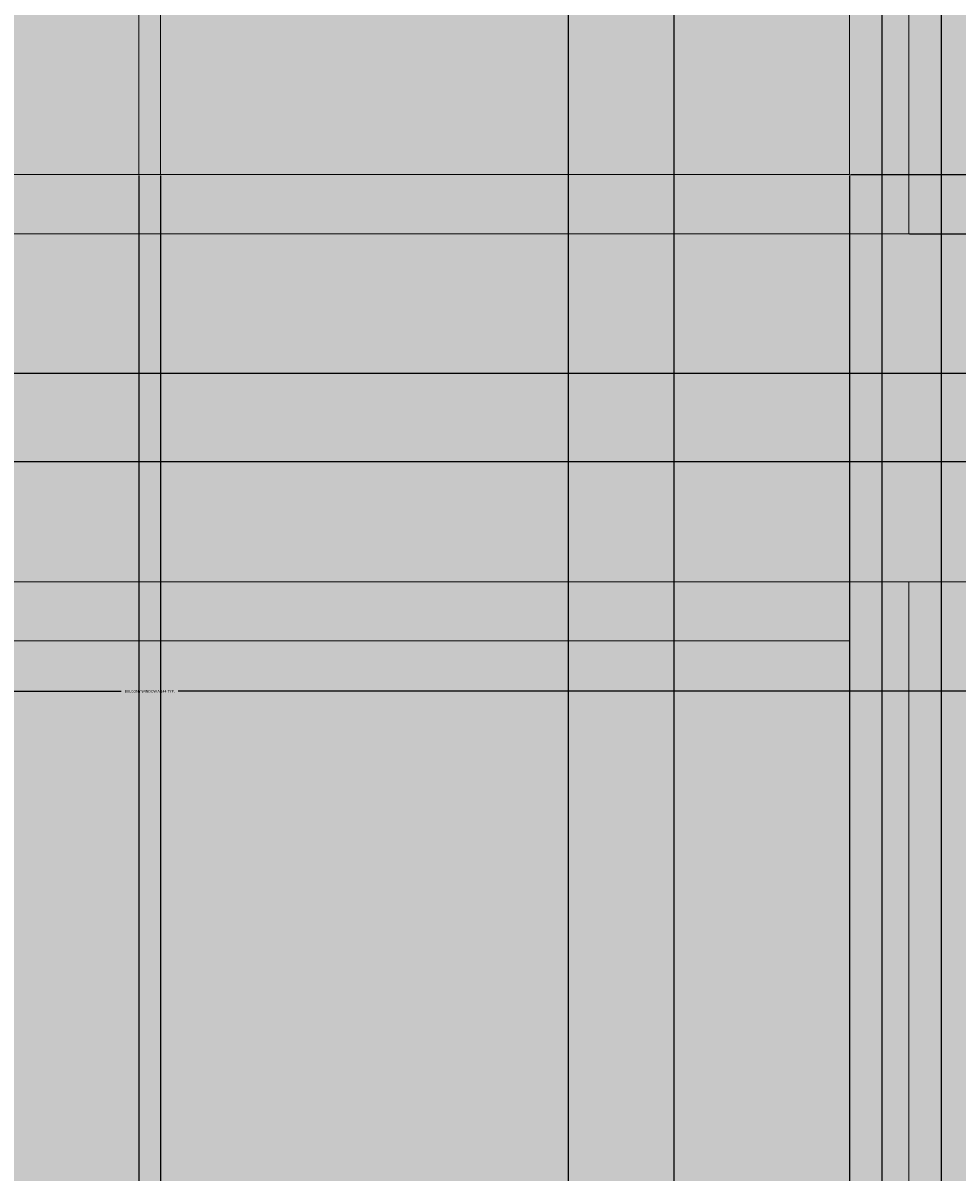
# Model space of a CAD drawing. Units: inches. Extents: x 3024 to 4744, y 1110 to 2100.
# Tile 21 of 29: x 3212 to 3275, y 1731 to 1809. Entities that reach past the tile are written whole.
import ezdxf

# ---------------------------------------------------------------- set-up
doc = ezdxf.new("R2010")
doc.units = ezdxf.units.IN
for name, color, linetype, lineweight in [('A-ANNO-DIMS', 2, 'Continuous', 18), ('A-ELEV', 7, 'Continuous', 25), ('A-ELEV-PATT', 252, 'Continuous', 13), ('A-GLAZ', 4, 'Continuous', 18)]:
    doc.layers.add(name, color=color, linetype=linetype, lineweight=lineweight)
doc.styles.get("Standard").update_dxf_attribs({"font": 'arial.ttf'})
doc.dimstyles.get("Standard").update_dxf_attribs({"dimtxt": 0.18, "dimasz": 0.18, "dimexe": 0.18, "dimexo": 0.0625, "dimgap": 0.09, "dimtad": 0, "dimtih": 1, "dimtoh": 1, "dimdec": 1, "dimzin": 0, "dimdsep": 46, "dimlunit": 3, "dimtxsty": 'Standard', "dimcen": 0.09, "dimadec": 0, "dimazin": 0, "dimtfac": 1, "dimtdec": 1, "dimtofl": 0, "dimtmove": 0, "dimatfit": 3, "dimfxl": 1, "dimtolj": 1, "dimtzin": 0, "dimarcsym": 0})

# ---------------------------------------------------------------- blocks, each defined once
blk = doc.blocks.new('WIN-BALCONY-A')
for p, q in [((3169.396, 1897.488), (3292.605, 1897.488)), ((3169.396, 1897.488), (3292.605, 1897.488)), ((3169.396, 1795.043), (3292.605, 1795.043)), ((3169.396, 1795.043), (3292.605, 1795.043))]:
    blk.add_line(p, q)
for points in [[(3148.969, 1897.488), (3148.969, 1905.611), (3292.605, 1905.611), (3292.605, 1897.488)], [(3148.969, 1897.488), (3148.969, 1905.611), (3292.605, 1905.611), (3292.605, 1897.488)], [(3292.605, 1795.043), (3292.605, 1785.611), (3148.969, 1785.611), (3148.969, 1795.043)], [(3292.605, 1795.043), (3292.605, 1785.611), (3148.969, 1785.611), (3148.969, 1795.043)]]:
    blk.add_lwpolyline(points)
for points in [[(3272.178, 1795.043), (3169.396, 1795.043), (3169.396, 1897.488), (3272.178, 1897.488)], [(3272.178, 1795.043), (3169.396, 1795.043), (3169.396, 1897.488), (3272.178, 1897.488)], [(3268.178, 1799.043), (3173.396, 1799.043), (3173.396, 1893.488), (3268.178, 1893.488)], [(3268.178, 1799.043), (3173.396, 1799.043), (3173.396, 1893.488), (3268.178, 1893.488)], [(3220.05, 1893.488), (3221.524, 1893.488), (3221.524, 1799.043), (3220.05, 1799.043)], [(3220.05, 1893.488), (3221.524, 1893.488), (3221.524, 1799.043), (3220.05, 1799.043)]]:
    blk.add_lwpolyline(points, close=True)
blk = doc.blocks.new('*D6')
at = {"layer": 'A-ANNO-DIMS', "color": 0, "lineweight": -2, "transparency": 16777216}
for p, q in [((3148.969, 1785.549), (3148.969, 1763.886)), ((3292.605, 1785.549), (3292.605, 1763.886)), ((3149.149, 1764.066), (3218.852, 1764.066)), ((3292.425, 1764.066), (3222.723, 1764.066))]:
    blk.add_line(p, q, dxfattribs=at)
at = {"layer": 'A-ANNO-DIMS', "color": 0, "transparency": 16777216}
for points in [[(3149.149, 1764.096), (3149.149, 1764.036), (3148.969, 1764.066)], [(3292.425, 1764.096), (3292.425, 1764.036), (3292.605, 1764.066)]]:
    blk.add_solid(points, dxfattribs=at)
at = {"layer": 'Defpoints', "color": 0, "transparency": 16777216}
for p in [(3148.969, 1785.611), (3292.605, 1785.611), (3292.605, 1764.066)]:
    blk.add_point(p, dxfattribs=at)
at = {"layer": 'A-ANNO-DIMS', "color": 0, "transparency": 16777216, "insert": (3220.787, 1764.066), "char_height": 0.18, "attachment_point": 5}
blk.add_mtext('\\A1;BALCONY WINDOW A 144 TYP.', dxfattribs=at)
blk = doc.blocks.new('*D64')
at = {"layer": 'A-ANNO-DIMS', "color": 0, "lineweight": -2, "transparency": 16777216}
for p, q in [((3069.794, 1241.497), (3069.794, 2100.438)), ((3741.151, 1241.497), (3741.151, 2100.438)), ((3069.974, 2100.258), (3405.078, 2100.258)), ((3740.971, 2100.258), (3405.866, 2100.258))]:
    blk.add_line(p, q, dxfattribs=at)
at = {"layer": 'A-ANNO-DIMS', "color": 0, "transparency": 16777216}
for points in [[(3069.974, 2100.288), (3069.974, 2100.228), (3069.794, 2100.258)], [(3740.971, 2100.288), (3740.971, 2100.228), (3741.151, 2100.258)]]:
    blk.add_solid(points, dxfattribs=at)
at = {"layer": 'Defpoints', "color": 0, "transparency": 16777216}
for p in [(3741.151, 2100.258), (3069.794, 1241.434), (3741.151, 1241.434)]:
    blk.add_point(p, dxfattribs=at)
at = {"layer": 'A-ANNO-DIMS', "color": 0, "transparency": 16777216, "insert": (3405.472, 2100.258), "char_height": 0.18, "attachment_point": 5}
blk.add_mtext('\\A1;671.4', dxfattribs=at)
blk = doc.blocks.new('*D91')
at = {"layer": 'A-ANNO-DIMS', "color": 0, "lineweight": -2, "transparency": 16777216}
for p, q in [((3173.396, 1798.981), (3173.396, 1109.931)), ((3220.05, 1798.981), (3220.05, 1109.931)), ((3173.576, 1110.111), (3196.325, 1110.111)), ((3219.87, 1110.111), (3197.121, 1110.111))]:
    blk.add_line(p, q, dxfattribs=at)
at = {"layer": 'A-ANNO-DIMS', "color": 0, "transparency": 16777216}
for points in [[(3173.576, 1110.141), (3173.576, 1110.081), (3173.396, 1110.111)], [(3219.87, 1110.141), (3219.87, 1110.081), (3220.05, 1110.111)]]:
    blk.add_solid(points, dxfattribs=at)
at = {"layer": 'Defpoints', "color": 0, "transparency": 16777216}
for p in [(3173.396, 1799.043), (3220.05, 1799.043), (3220.05, 1110.111)]:
    blk.add_point(p, dxfattribs=at)
at = {"layer": 'A-ANNO-DIMS', "color": 0, "transparency": 16777216, "insert": (3196.723, 1110.111), "char_height": 0.18, "attachment_point": 5}
blk.add_mtext('\\A1;46.65', dxfattribs=at)
blk = doc.blocks.new('*D92')
at = {"layer": 'A-ANNO-DIMS', "color": 0, "lineweight": -2, "transparency": 16777216}
for p, q in [((3220.05, 1798.981), (3220.05, 1109.931)), ((3221.524, 1798.981), (3221.524, 1109.931)), ((3220.23, 1110.111), (3220.472, 1110.111)), ((3221.344, 1110.111), (3221.103, 1110.111))]:
    blk.add_line(p, q, dxfattribs=at)
at = {"layer": 'A-ANNO-DIMS', "color": 0, "transparency": 16777216}
for points in [[(3220.23, 1110.141), (3220.23, 1110.081), (3220.05, 1110.111)], [(3221.344, 1110.141), (3221.344, 1110.081), (3221.524, 1110.111)]]:
    blk.add_solid(points, dxfattribs=at)
at = {"layer": 'Defpoints', "color": 0, "transparency": 16777216}
for p in [(3220.05, 1799.043), (3221.524, 1799.043), (3221.524, 1110.111)]:
    blk.add_point(p, dxfattribs=at)
at = {"layer": 'A-ANNO-DIMS', "color": 0, "transparency": 16777216, "insert": (3220.787, 1110.111), "char_height": 0.18, "attachment_point": 5}
blk.add_mtext('\\A1;1.47', dxfattribs=at)
blk = doc.blocks.new('*D93')
at = {"layer": 'A-ANNO-DIMS', "color": 0, "lineweight": -2, "transparency": 16777216}
for p, q in [((3221.524, 1798.981), (3221.524, 1109.931)), ((3268.178, 1798.981), (3268.178, 1109.931)), ((3221.704, 1110.111), (3244.453, 1110.111)), ((3267.998, 1110.111), (3245.249, 1110.111))]:
    blk.add_line(p, q, dxfattribs=at)
at = {"layer": 'A-ANNO-DIMS', "color": 0, "transparency": 16777216}
for points in [[(3221.704, 1110.141), (3221.704, 1110.081), (3221.524, 1110.111)], [(3267.998, 1110.141), (3267.998, 1110.081), (3268.178, 1110.111)]]:
    blk.add_solid(points, dxfattribs=at)
at = {"layer": 'Defpoints', "color": 0, "transparency": 16777216}
for p in [(3221.524, 1799.043), (3268.178, 1799.043), (3268.178, 1110.111)]:
    blk.add_point(p, dxfattribs=at)
at = {"layer": 'A-ANNO-DIMS', "color": 0, "transparency": 16777216, "insert": (3244.851, 1110.111), "char_height": 0.18, "attachment_point": 5}
blk.add_mtext('\\A1;46.65', dxfattribs=at)
blk = doc.blocks.new('*D100')
at = {"layer": 'A-ANNO-DIMS', "color": 0, "lineweight": -2, "transparency": 16777216}
for p, q in [((3268.241, 1799.043), (3786.831, 1799.043)), ((3786.651, 1798.863), (3786.651, 1797.225)), ((3786.651, 1795.223), (3786.651, 1796.861)), ((3272.241, 1795.043), (3786.831, 1795.043))]:
    blk.add_line(p, q, dxfattribs=at)
at = {"layer": 'A-ANNO-DIMS', "color": 0, "transparency": 16777216}
for points in [[(3786.621, 1798.863), (3786.681, 1798.863), (3786.651, 1799.043)], [(3786.621, 1795.223), (3786.681, 1795.223), (3786.651, 1795.043)]]:
    blk.add_solid(points, dxfattribs=at)
at = {"layer": 'Defpoints', "color": 0, "transparency": 16777216}
for p in [(3268.178, 1799.043), (3786.651, 1799.043), (3272.178, 1795.043)]:
    blk.add_point(p, dxfattribs=at)
at = {"layer": 'A-ANNO-DIMS', "color": 0, "transparency": 16777216, "insert": (3786.651, 1797.043), "char_height": 0.18, "attachment_point": 5}
blk.add_mtext('\\A1;4.00', dxfattribs=at)
blk = doc.blocks.new('*D101')
at = {"layer": 'A-ANNO-DIMS', "color": 0, "lineweight": -2, "transparency": 16777216}
for p, q in [((3268.241, 1893.488), (3786.831, 1893.488)), ((3786.651, 1893.308), (3786.651, 1846.447)), ((3786.651, 1799.223), (3786.651, 1846.084)), ((3268.241, 1799.043), (3786.831, 1799.043))]:
    blk.add_line(p, q, dxfattribs=at)
at = {"layer": 'A-ANNO-DIMS', "color": 0, "transparency": 16777216}
for points in [[(3786.621, 1893.308), (3786.681, 1893.308), (3786.651, 1893.488)], [(3786.621, 1799.223), (3786.681, 1799.223), (3786.651, 1799.043)]]:
    blk.add_solid(points, dxfattribs=at)
at = {"layer": 'Defpoints', "color": 0, "transparency": 16777216}
for p in [(3268.178, 1893.488), (3786.651, 1893.488), (3268.178, 1799.043)]:
    blk.add_point(p, dxfattribs=at)
at = {"layer": 'A-ANNO-DIMS', "color": 0, "transparency": 16777216, "insert": (3786.651, 1846.265), "char_height": 0.18, "attachment_point": 5}
blk.add_mtext('\\A1;94.44', dxfattribs=at)
blk = doc.blocks.new('*D107')
at = {"layer": 'A-ANNO-DIMS', "color": 0, "lineweight": -2, "transparency": 16777216}
for p, q in [((3174.161, 1271.674), (3174.161, 2100.438)), ((3270.388, 1271.674), (3270.388, 2100.438)), ((3174.341, 2100.258), (3221.881, 2100.258)), ((3270.208, 2100.258), (3222.668, 2100.258))]:
    blk.add_line(p, q, dxfattribs=at)
at = {"layer": 'A-ANNO-DIMS', "color": 0, "transparency": 16777216}
for points in [[(3174.341, 2100.288), (3174.341, 2100.228), (3174.161, 2100.258)], [(3270.208, 2100.288), (3270.208, 2100.228), (3270.388, 2100.258)]]:
    blk.add_solid(points, dxfattribs=at)
at = {"layer": 'Defpoints', "color": 0, "transparency": 16777216}
for p in [(3270.388, 2100.258), (3174.161, 1271.611), (3270.388, 1271.611)]:
    blk.add_point(p, dxfattribs=at)
at = {"layer": 'A-ANNO-DIMS', "color": 0, "transparency": 16777216, "insert": (3222.274, 2100.258), "char_height": 0.18, "attachment_point": 5}
blk.add_mtext('\\A1;96.23', dxfattribs=at)
blk = doc.blocks.new('*D108')
at = {"layer": 'A-ANNO-DIMS', "color": 0, "lineweight": -2, "transparency": 16777216}
for p, q in [((3270.388, 1271.674), (3270.388, 2100.438)), ((3274.388, 1275.674), (3274.388, 2100.438)), ((3270.568, 2100.258), (3272.061, 2100.258)), ((3274.208, 2100.258), (3272.715, 2100.258))]:
    blk.add_line(p, q, dxfattribs=at)
at = {"layer": 'A-ANNO-DIMS', "color": 0, "transparency": 16777216}
for points in [[(3270.568, 2100.288), (3270.568, 2100.228), (3270.388, 2100.258)], [(3274.208, 2100.288), (3274.208, 2100.228), (3274.388, 2100.258)]]:
    blk.add_solid(points, dxfattribs=at)
at = {"layer": 'Defpoints', "color": 0, "transparency": 16777216}
for p in [(3274.388, 2100.258), (3274.388, 1275.611), (3270.388, 1271.611)]:
    blk.add_point(p, dxfattribs=at)
at = {"layer": 'A-ANNO-DIMS', "color": 0, "transparency": 16777216, "insert": (3272.388, 2100.258), "char_height": 0.18, "attachment_point": 5}
blk.add_mtext('\\A1;4.00', dxfattribs=at)
blk = doc.blocks.new('*D126')
at = {"layer": 'A-ANNO-DIMS', "color": 0, "lineweight": -2, "transparency": 16777216}
for p, q in [((3249.143, 1256.29), (3249.143, 2100.438)), ((3256.29, 1256.29), (3256.29, 2100.438)), ((3249.323, 2100.258), (3252.324, 2100.258)), ((3256.11, 2100.258), (3253.11, 2100.258))]:
    blk.add_line(p, q, dxfattribs=at)
at = {"layer": 'A-ANNO-DIMS', "color": 0, "transparency": 16777216}
for points in [[(3249.323, 2100.288), (3249.323, 2100.228), (3249.143, 2100.258)], [(3256.11, 2100.288), (3256.11, 2100.228), (3256.29, 2100.258)]]:
    blk.add_solid(points, dxfattribs=at)
at = {"layer": 'Defpoints', "color": 0, "transparency": 16777216}
for p in [(3256.29, 2100.258), (3249.143, 1256.228), (3256.29, 1256.228)]:
    blk.add_point(p, dxfattribs=at)
at = {"layer": 'A-ANNO-DIMS', "color": 0, "transparency": 16777216, "insert": (3252.717, 2100.258), "char_height": 0.18, "attachment_point": 5}
blk.add_mtext('\\A1;7.147', dxfattribs=at)

msp = doc.modelspace()

# ---------------------------------------------------------------- hatches: boundary and pattern name
at = {"layer": 'A-ELEV-PATT'}
h = msp.add_hatch(color=256, dxfattribs=at)
h.dxf.hatch_style = 1
h.paths.add_polyline_path([(3491.8271, 2054.7584), (3320.5658, 2054.7584), (3320.5658, 2043.5286), (3491.8271, 2043.5286)])
h.paths.add_polyline_path([(3292.6051, 1905.6112), (3148.9694, 1905.6112), (3148.9694, 1897.4879), (3169.3964, 1897.4879), (3292.6051, 1897.4879)])
h.paths.add_polyline_path([(3292.6051, 1795.0431), (3169.3964, 1795.0431), (3148.9694, 1795.0431), (3148.9694, 1785.6112), (3292.6051, 1785.6112)])
h.paths.add_polyline_path([(3292.6051, 1779.6112), (3148.9694, 1779.6112), (3148.9694, 1771.4879), (3169.3964, 1771.4879), (3292.6051, 1771.4879)])
h.paths.add_polyline_path([(3292.6051, 1669.0431), (3169.3964, 1669.0431), (3148.9694, 1669.0431), (3148.9694, 1659.6112), (3292.6051, 1659.6112)])
h.paths.add_polyline_path([(3292.6051, 1653.6112), (3148.9694, 1653.6112), (3148.9694, 1645.4879), (3169.3964, 1645.4879), (3292.6051, 1645.4879)])
h.paths.add_polyline_path([(3292.6051, 1543.0431), (3169.3964, 1543.0431), (3148.9694, 1543.0431), (3148.9694, 1533.6112), (3292.6051, 1533.6112)])
h.paths.add_polyline_path([(3292.6051, 1527.6112), (3148.9694, 1527.6112), (3148.9694, 1519.4879), (3169.3964, 1519.4879), (3292.6051, 1519.4879)])
h.paths.add_polyline_path([(3292.6051, 1401.6112), (3148.9694, 1401.6112), (3148.9694, 1393.4879), (3169.3964, 1393.4879), (3292.6051, 1393.4879)])
h.paths.add_polyline_path([(3292.6051, 1417.0431), (3169.3964, 1417.0431), (3148.9694, 1417.0431), (3148.9694, 1407.6112), (3292.6051, 1407.6112)])
h.paths.add_polyline_path([(3292.6051, 1291.0431), (3169.3964, 1291.0431), (3148.9694, 1291.0431), (3148.9694, 1281.6112), (3292.6051, 1281.6112)])
h.paths.add_polyline_path([(3654.037, 1165.0431), (3530.8283, 1165.0431), (3510.4013, 1165.0431), (3510.4013, 1155.6112), (3654.037, 1155.6112)])
h.paths.add_polyline_path([(3654.037, 1275.6112), (3510.4013, 1275.6112), (3510.4013, 1267.4879), (3530.8283, 1267.4879), (3654.037, 1267.4879)])
h.paths.add_polyline_path([(3654.037, 1291.0431), (3530.8283, 1291.0431), (3510.4013, 1291.0431), (3510.4013, 1281.6112), (3654.037, 1281.6112)])
h.paths.add_polyline_path([(3654.037, 1417.0431), (3530.8283, 1417.0431), (3510.4013, 1417.0431), (3510.4013, 1407.6112), (3654.037, 1407.6112)])
h.paths.add_polyline_path([(3654.037, 1401.6112), (3510.4013, 1401.6112), (3510.4013, 1393.4879), (3530.8283, 1393.4879), (3654.037, 1393.4879)])
h.paths.add_polyline_path([(3654.037, 1543.0431), (3530.8283, 1543.0431), (3510.4013, 1543.0431), (3510.4013, 1533.6112), (3654.037, 1533.6112)])
h.paths.add_polyline_path([(3654.037, 1527.6112), (3510.4013, 1527.6112), (3510.4013, 1519.4879), (3530.8283, 1519.4879), (3654.037, 1519.4879)])
h.paths.add_polyline_path([(3654.037, 1653.6112), (3510.4013, 1653.6112), (3510.4013, 1645.4879), (3530.8283, 1645.4879), (3654.037, 1645.4879)])
h.paths.add_polyline_path([(3654.037, 1669.0431), (3530.8283, 1669.0431), (3510.4013, 1669.0431), (3510.4013, 1659.6112), (3654.037, 1659.6112)])
h.paths.add_polyline_path([(3654.037, 1779.6112), (3510.4013, 1779.6112), (3510.4013, 1771.4879), (3530.8283, 1771.4879), (3654.037, 1771.4879)])
h.paths.add_polyline_path([(3654.037, 1795.0431), (3530.8283, 1795.0431), (3510.4013, 1795.0431), (3510.4013, 1785.6112), (3654.037, 1785.6112)])
h.paths.add_polyline_path([(3654.037, 1905.6112), (3510.4013, 1905.6112), (3510.4013, 1897.4879), (3530.8283, 1897.4879), (3654.037, 1897.4879)])
h = msp.add_hatch(color=256, dxfattribs=at)
h.dxf.hatch_style = 1
h.paths.add_polyline_path([(3221.5241, 2019.4879), (3220.0505, 2019.4879), (3220.0505, 1925.0431), (3221.5241, 1925.0431)], flags=0)
h.paths.add_polyline_path([(3221.5241, 2019.4879), (3221.5241, 1925.0431), (3220.0505, 1925.0431), (3220.0505, 2019.4879)], flags=0)
h.paths.add_polyline_path([(3221.5241, 1893.4879), (3220.0505, 1893.4879), (3220.0505, 1799.0431), (3221.5241, 1799.0431)])
h = msp.add_hatch(color=256, dxfattribs=at)
h.dxf.hatch_style = 1
h.paths.add_polyline_path([(3329.7033, 1407.6112), (3105.4722, 1407.6112), (3105.4722, 1401.6112), (3329.7033, 1401.6112)])
h.paths.add_polyline_path([(3329.7033, 1281.6112), (3105.4722, 1281.6112), (3105.4722, 1275.6112), (3112.3838, 1275.6112), (3329.7033, 1275.6112)])
h.paths.add_polyline_path([(3329.7033, 1533.6112), (3105.4722, 1533.6112), (3105.4722, 1527.6112), (3329.7033, 1527.6112)])
h.paths.add_polyline_path([(3329.7033, 1659.6112), (3105.4722, 1659.6112), (3105.4722, 1653.6112), (3329.7033, 1653.6112)])
h.paths.add_polyline_path([(3329.7033, 1785.6112), (3105.4722, 1785.6112), (3105.4722, 1779.6112), (3329.7033, 1779.6112)])
h.paths.add_polyline_path([(3329.7033, 1911.6112), (3105.4722, 1911.6112), (3095.7158, 1911.6112), (3095.7158, 1905.6112), (3329.7033, 1905.6112)])
h.paths.add_polyline_path([(3715.2286, 1911.6112), (3705.4722, 1911.6112), (3705.4722, 1905.6112), (3715.2286, 1905.6112)])
h.paths.add_polyline_path([(3688.5588, 1911.6112), (3481.2411, 1911.6112), (3481.2411, 1905.6112), (3688.5588, 1905.6112)])
h = msp.add_hatch(color=256, dxfattribs=at)
h.dxf.hatch_style = 1
h.paths.add_polyline_path([(3169.3964, 1897.4879), (3160.8586, 1897.4879), (3160.8586, 1806.8674), (3163.5269, 1806.8674), (3163.5269, 1795.0431), (3169.3964, 1795.0431)])
h.paths.add_polyline_path([(3280.716, 1897.4879), (3272.1781, 1897.4879), (3272.1781, 1795.0431), (3276.5094, 1795.0431), (3276.5094, 1806.8674), (3280.716, 1806.8674)])
h.paths.add_polyline_path([(3280.716, 1771.4879), (3272.1781, 1771.4879), (3272.1781, 1669.0431), (3276.5094, 1669.0431), (3276.5094, 1680.8674), (3280.716, 1680.8674)])
h.paths.add_polyline_path([(3169.3964, 1771.4879), (3160.8586, 1771.4879), (3160.8586, 1680.8674), (3163.5269, 1680.8674), (3163.5269, 1669.0431), (3169.3964, 1669.0431)])
h.paths.add_polyline_path([(3169.3964, 1645.4879), (3160.8586, 1645.4879), (3160.8586, 1554.8674), (3163.5269, 1554.8674), (3163.5269, 1543.0431), (3169.3964, 1543.0431)])
h.paths.add_polyline_path([(3280.716, 1645.4879), (3272.1781, 1645.4879), (3272.1781, 1543.0431), (3276.5094, 1543.0431), (3276.5094, 1554.8674), (3280.716, 1554.8674)])
h.paths.add_polyline_path([(3169.3964, 1519.4879), (3160.8586, 1519.4879), (3160.8586, 1428.8674), (3163.5269, 1428.8674), (3163.5269, 1417.0431), (3169.3964, 1417.0431)])
h.paths.add_polyline_path([(3280.716, 1519.4879), (3272.1781, 1519.4879), (3272.1781, 1417.0431), (3276.5094, 1417.0431), (3276.5094, 1428.8674), (3280.716, 1428.8674)])
h.paths.add_polyline_path([(3169.3964, 1393.4879), (3160.8586, 1393.4879), (3160.8586, 1302.8674), (3163.5269, 1302.8674), (3163.5269, 1291.0431), (3169.3964, 1291.0431)])
h.paths.add_polyline_path([(3280.716, 1393.4879), (3272.1781, 1393.4879), (3272.1781, 1291.0431), (3276.5094, 1291.0431), (3276.5094, 1302.8674), (3280.716, 1302.8674)])
h.paths.add_polyline_path([(3642.1479, 1267.4879), (3633.61, 1267.4879), (3633.61, 1165.0431), (3637.9413, 1165.0431), (3637.9413, 1176.8674), (3642.1479, 1176.8674)])
h.paths.add_polyline_path([(3530.8283, 1267.4879), (3522.2905, 1267.4879), (3522.2905, 1176.8674), (3524.9588, 1176.8674), (3524.9588, 1165.0431), (3530.8283, 1165.0431)])
h.paths.add_polyline_path([(3642.1479, 1393.4879), (3633.61, 1393.4879), (3633.61, 1291.0431), (3637.9413, 1291.0431), (3637.9413, 1302.8674), (3642.1479, 1302.8674)])
h.paths.add_polyline_path([(3530.8283, 1393.4879), (3522.2905, 1393.4879), (3522.2905, 1302.8674), (3524.9588, 1302.8674), (3524.9588, 1291.0431), (3530.8283, 1291.0431)])
h.paths.add_polyline_path([(3530.8283, 1519.4879), (3522.2905, 1519.4879), (3522.2905, 1428.8674), (3524.9588, 1428.8674), (3524.9588, 1417.0431), (3530.8283, 1417.0431)])
h.paths.add_polyline_path([(3642.1479, 1519.4879), (3633.61, 1519.4879), (3633.61, 1417.0431), (3637.9413, 1417.0431), (3637.9413, 1428.8674), (3642.1479, 1428.8674)])
h.paths.add_polyline_path([(3530.8283, 1645.4879), (3522.2905, 1645.4879), (3522.2905, 1554.8674), (3524.9588, 1554.8674), (3524.9588, 1543.0431), (3530.8283, 1543.0431)])
h.paths.add_polyline_path([(3642.1479, 1645.4879), (3633.61, 1645.4879), (3633.61, 1543.0431), (3637.9413, 1543.0431), (3637.9413, 1554.8674), (3642.1479, 1554.8674)])
h.paths.add_polyline_path([(3642.1479, 1771.4879), (3633.61, 1771.4879), (3633.61, 1669.0431), (3637.9413, 1669.0431), (3637.9413, 1680.8674), (3642.1479, 1680.8674)])
h.paths.add_polyline_path([(3530.8283, 1771.4879), (3522.2905, 1771.4879), (3522.2905, 1680.8674), (3524.9588, 1680.8674), (3524.9588, 1669.0431), (3530.8283, 1669.0431)])
h.paths.add_polyline_path([(3530.8283, 1897.4879), (3522.2905, 1897.4879), (3522.2905, 1806.8674), (3524.9588, 1806.8674), (3524.9588, 1795.0431), (3530.8283, 1795.0431)])
h.paths.add_polyline_path([(3642.1479, 1897.4879), (3633.61, 1897.4879), (3633.61, 1795.0431), (3637.9413, 1795.0431), (3637.9413, 1806.8674), (3642.1479, 1806.8674)])
h = msp.add_hatch(color=256, dxfattribs=at)
h.dxf.hatch_style = 1
h.paths.add_polyline_path([(3221.5241, 1893.4879), (3220.0505, 1893.4879), (3220.0505, 1799.0431), (3221.5241, 1799.0431)], flags=0)
h.paths.add_polyline_path([(3272.1781, 1897.4879), (3169.3964, 1897.4879), (3169.3964, 1795.0431), (3272.1781, 1795.0431)])
h.paths.add_polyline_path([(3268.1781, 1893.4879), (3268.1781, 1799.0431), (3173.3964, 1799.0431), (3173.3964, 1893.4879)], flags=16)
h.paths.add_polyline_path([(3221.5241, 1893.4879), (3221.5241, 1799.0431), (3220.0505, 1799.0431), (3220.0505, 1893.4879)], flags=0)
h = msp.add_hatch(color=256, dxfattribs=at)
h.dxf.hatch_style = 1
h.paths.add_polyline_path([(3220.0505, 1893.4879), (3173.3964, 1893.4879), (3173.3964, 1799.0431), (3220.0505, 1799.0431)])
h.paths.add_polyline_path([(3268.1781, 1893.4879), (3221.5241, 1893.4879), (3221.5241, 1799.0431), (3268.1781, 1799.0431)])
h.paths.add_polyline_path([(3581.4824, 1893.4879), (3534.8283, 1893.4879), (3534.8283, 1799.0431), (3581.4824, 1799.0431)])
h.paths.add_polyline_path([(3629.61, 1893.4879), (3582.956, 1893.4879), (3582.956, 1799.0431), (3629.61, 1799.0431)])
h.paths.add_polyline_path([(3581.4824, 1767.4879), (3534.8283, 1767.4879), (3534.8283, 1673.0431), (3581.4824, 1673.0431)])
h.paths.add_polyline_path([(3629.61, 1767.4879), (3582.956, 1767.4879), (3582.956, 1673.0431), (3629.61, 1673.0431)])
h.paths.add_polyline_path([(3581.4824, 1641.4879), (3534.8283, 1641.4879), (3534.8283, 1547.0431), (3581.4824, 1547.0431)])
h.paths.add_polyline_path([(3629.61, 1641.4879), (3582.956, 1641.4879), (3582.956, 1547.0431), (3629.61, 1547.0431)])
h.paths.add_polyline_path([(3629.61, 1515.4879), (3582.956, 1515.4879), (3582.956, 1421.0431), (3629.61, 1421.0431)])
h.paths.add_polyline_path([(3581.4824, 1515.4879), (3534.8283, 1515.4879), (3534.8283, 1421.0431), (3581.4824, 1421.0431)])
h.paths.add_polyline_path([(3629.61, 1389.4879), (3582.956, 1389.4879), (3582.956, 1295.0431), (3629.61, 1295.0431)])
h.paths.add_polyline_path([(3581.4824, 1389.4879), (3534.8283, 1389.4879), (3534.8283, 1295.0431), (3581.4824, 1295.0431)])
h.paths.add_polyline_path([(3629.61, 1263.4879), (3582.956, 1263.4879), (3582.956, 1169.0431), (3629.61, 1169.0431)])
h.paths.add_polyline_path([(3581.4824, 1263.4879), (3534.8283, 1263.4879), (3534.8283, 1169.0431), (3581.4824, 1169.0431)])
h.paths.add_polyline_path([(3220.0505, 1389.4879), (3173.3964, 1389.4879), (3173.3964, 1295.0431), (3220.0505, 1295.0431)])
h.paths.add_polyline_path([(3268.1781, 1389.4879), (3221.5241, 1389.4879), (3221.5241, 1295.0431), (3268.1781, 1295.0431)])
h.paths.add_polyline_path([(3220.0505, 1515.4879), (3173.3964, 1515.4879), (3173.3964, 1421.0431), (3220.0505, 1421.0431)])
h.paths.add_polyline_path([(3268.1781, 1515.4879), (3221.5241, 1515.4879), (3221.5241, 1421.0431), (3268.1781, 1421.0431)])
h.paths.add_polyline_path([(3220.0505, 1767.4879), (3173.3964, 1767.4879), (3173.3964, 1673.0431), (3220.0505, 1673.0431)])
h.paths.add_polyline_path([(3268.1781, 1767.4879), (3221.5241, 1767.4879), (3221.5241, 1673.0431), (3268.1781, 1673.0431)])
h.paths.add_polyline_path([(3220.0505, 1641.4879), (3173.3964, 1641.4879), (3173.3964, 1547.0431), (3220.0505, 1547.0431)])
h.paths.add_polyline_path([(3268.1781, 1641.4879), (3221.5241, 1641.4879), (3221.5241, 1547.0431), (3268.1781, 1547.0431)])
h = msp.add_hatch(color=256, dxfattribs=at)
h.dxf.hatch_style = 1
h.paths.add_polyline_path([(3221.5241, 1893.4879), (3220.0505, 1893.4879), (3220.0505, 1799.0431), (3221.5241, 1799.0431)], flags=0)
h.paths.add_polyline_path([(3221.5241, 1893.4879), (3221.5241, 1799.0431), (3220.0505, 1799.0431), (3220.0505, 1893.4879)], flags=0)
h.paths.add_polyline_path([(3221.5241, 1767.4879), (3220.0505, 1767.4879), (3220.0505, 1673.0431), (3221.5241, 1673.0431)])
h = msp.add_hatch(color=256, dxfattribs=at)
h.dxf.hatch_style = 1
h.paths.add_polyline_path([(3221.5241, 1767.4879), (3220.0505, 1767.4879), (3220.0505, 1673.0431), (3221.5241, 1673.0431)], flags=0)
h.paths.add_polyline_path([(3272.1781, 1771.4879), (3169.3964, 1771.4879), (3169.3964, 1669.0431), (3272.1781, 1669.0431)])
h.paths.add_polyline_path([(3268.1781, 1767.4879), (3268.1781, 1673.0431), (3173.3964, 1673.0431), (3173.3964, 1767.4879)], flags=16)
h.paths.add_polyline_path([(3221.5241, 1767.4879), (3221.5241, 1673.0431), (3220.0505, 1673.0431), (3220.0505, 1767.4879)], flags=0)
h = msp.add_hatch(color=256, dxfattribs=at)
h.dxf.hatch_style = 1
h.paths.add_polyline_path([(3221.5241, 1767.4879), (3220.0505, 1767.4879), (3220.0505, 1673.0431), (3221.5241, 1673.0431)], flags=0)
h.paths.add_polyline_path([(3221.5241, 1767.4879), (3221.5241, 1673.0431), (3220.0505, 1673.0431), (3220.0505, 1767.4879)], flags=0)
h.paths.add_polyline_path([(3221.5241, 1641.4879), (3220.0505, 1641.4879), (3220.0505, 1547.0431), (3221.5241, 1547.0431)])

# ---------------------------------------------------------------- linework, layer by layer
at = {"layer": 'A-ELEV'}
for p, q in [((3105.4722, 1785.6112), (3329.7033, 1785.6112)), ((3105.4722, 1785.6112), (3329.7033, 1785.6112)), ((3329.7033, 1779.6112), (3105.4722, 1779.6112)), ((3329.7033, 1779.6112), (3105.4722, 1779.6112))]:
    msp.add_line(p, q, dxfattribs=at)

# ---------------------------------------------------------------- block references
at = {"layer": 'A-GLAZ'}
for p in [(0, 0), (0, -126)]:
    msp.add_blockref('WIN-BALCONY-A', p, dxfattribs=at)

# ---------------------------------------------------------------- dimensions: what is measured, and where the dimension line sits
at = {"layer": 'A-ANNO-DIMS'}
for base, p1, p2, override, picture, middle in [((3741.1507, 2100.2584), (3069.7937, 1241.4341), (3741.1507, 1241.4341), {"dimdec": 1, "dimlfac": 1, "dimrnd": 0, "dimzin": 0, "dimdsep": 46, "dimlunit": 2}, '*D64', (3405.4722, 2100.2584)), ((3270.3877, 2100.2584), (3174.1608, 1271.6112), (3270.3877, 1271.6112), {"dimdec": 2, "dimlfac": 1, "dimrnd": 0, "dimzin": 0, "dimdsep": 46, "dimlunit": 2}, '*D107', (3222.2743, 2100.2584)), ((3256.2899, 2100.2584), (3249.1433, 1256.2276), (3256.2899, 1256.2276), {"dimdec": 3, "dimlfac": 1, "dimrnd": 0, "dimzin": 0, "dimdsep": 46, "dimlunit": 2}, '*D126', (3252.7166, 2100.2584)), ((3274.3877, 2100.2584), (3270.3877, 1271.6112), (3274.3877, 1275.6112), {"dimdec": 2, "dimlfac": 1, "dimrnd": 0, "dimzin": 0, "dimdsep": 46, "dimlunit": 2}, '*D108', (3272.3877, 2100.2584)), ((3220.0505, 1110.1112), (3173.3964, 1799.0431), (3220.0505, 1799.0431), {"dimdec": 2, "dimlfac": 1, "dimrnd": 0, "dimzin": 0, "dimdsep": 46, "dimlunit": 2}, '*D91', (3196.7234, 1110.1112)), ((3221.5241, 1110.1112), (3220.0505, 1799.0431), (3221.5241, 1799.0431), {"dimdec": 2, "dimlfac": 1, "dimrnd": 0, "dimzin": 0, "dimdsep": 46, "dimlunit": 2}, '*D92', (3220.7873, 1110.1112)), ((3268.1781, 1110.1112), (3221.5241, 1799.0431), (3268.1781, 1799.0431), {"dimdec": 2, "dimlfac": 1, "dimrnd": 0, "dimzin": 0, "dimdsep": 46, "dimlunit": 2}, '*D93', (3244.8511, 1110.1112))]:
    dim = msp.add_linear_dim(base=base, p1=p1, p2=p2, dimstyle='Standard', override=override, dxfattribs=at)
    dim.commit()
    dim.dimension.update_dxf_attribs({"geometry": picture, "text_midpoint": middle})
for base, p1, p2, picture, middle in [((3786.6507, 1893.4879), (3268.1781, 1799.0431), (3268.1781, 1893.4879), '*D101', (3786.6507, 1846.2655)), ((3786.6507, 1799.0431), (3272.1781, 1795.0431), (3268.1781, 1799.0431), '*D100', (3786.6507, 1797.0431))]:
    dim = msp.add_linear_dim(base=base, p1=p1, p2=p2, angle=90, dimstyle='Standard', override={"dimdec": 2, "dimlfac": 1, "dimrnd": 0, "dimzin": 0, "dimdsep": 46, "dimlunit": 2}, dxfattribs=at)
    dim.commit()
    dim.dimension.update_dxf_attribs({"geometry": picture, "text_midpoint": middle})
dim = msp.add_linear_dim(base=(3292.6051, 1764.0658), p1=(3148.9694, 1785.6112), p2=(3292.6051, 1785.6112), text='BALCONY WINDOW A <> TYP.', dimstyle='Standard', override={"dimdec": 0, "dimrnd": 0, "dimzin": 0, "dimlunit": 2}, dxfattribs=at)
dim.commit()
dim.dimension.update_dxf_attribs({"geometry": '*D6', "text_midpoint": (3220.7873, 1764.0658)})

doc.saveas('drawing.dxf')
